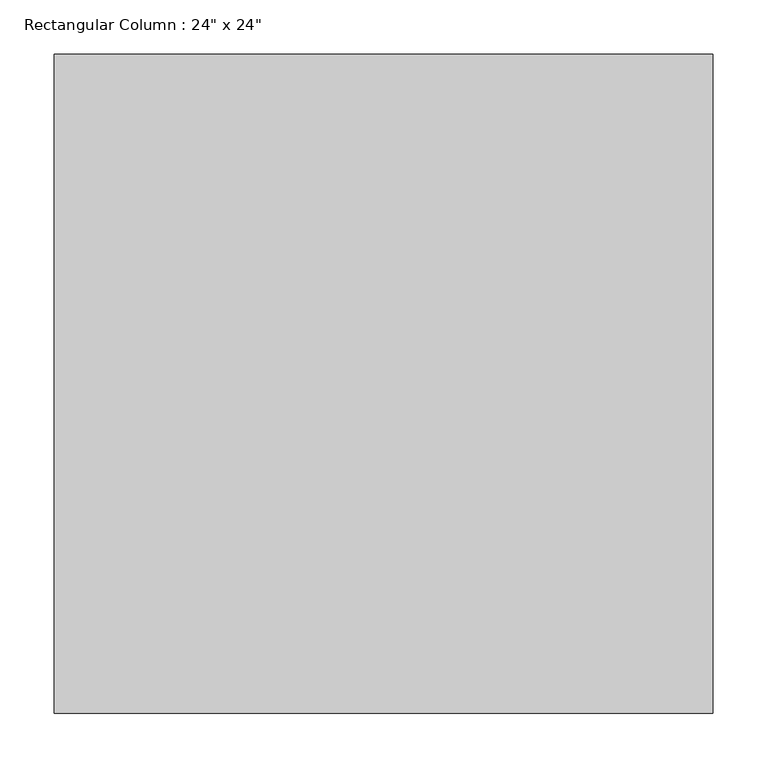
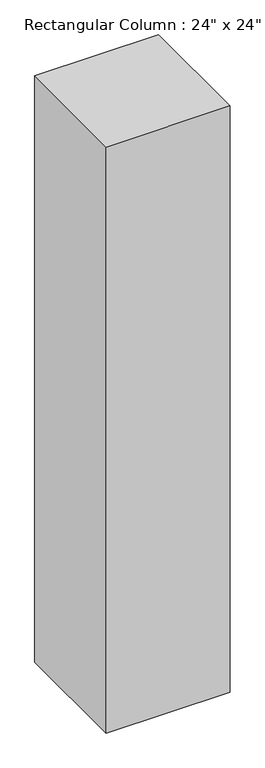
"""IFC4 building model written with IfcOpenShell, lengths in millimetres: column geometry."""

from ifc_helpers import new_model, si_unit, frame, origin, place, context, project, spatial, polyline, outline, extrude, source, transform, mapped, element, save


def column_08700e81(model_context):
    return source(origin(), model_context, "Body", "SweptSolid", [
        extrude(outline(polyline([(304.8, 304.8), (304.8, -304.8), (-304.8, -304.8), (-304.8, 304.8), (304.8, 304.8)])), frame((0.0, 0.0, 9601.2), z_axis=(0.0, 0.0, 1.0), x_axis=(1.0, 0.0, 0.0)), (0.0, 0.0, 1.0), 3048.0),
    ])


if __name__ == "__main__":
    model = new_model("IFC4")
    model_context = context("Model", 3, world=origin())
    ifc_project = project(units=[si_unit("LENGTHUNIT", "METRE", prefix="MILLI")], contexts=[model_context])
    site = spatial("IfcSite", under=ifc_project)
    building = spatial("IfcBuilding", under=site)
    placement = place(None, origin())
    column_shape = column_08700e81(model_context)
    element("IfcColumn", 1, ObjectType="Rectangular Column : 24\" x 24\"", at=placement, inside=building, context=model_context, shape_type="MappedRepresentation", body=[
        mapped(column_shape, transform((0.0, 0.0, 0.0), x_axis=(1.0, 0.0, 0.0), y_axis=(0.0, 1.0, 0.0), z_axis=(0.0, 0.0, 1.0))),
    ])
    save(model, "model.ifc")

# Revit data of these elements
# Type "Rectangular Column : 24\" x 24\""
#   Assembly Code = "B1010200"
#   Depth = 2' - 0"
#   Offset Base = 0' - 0"
#   Offset Top = 0' - 0"
#   Width = 2' - 0"
#   Material = none
